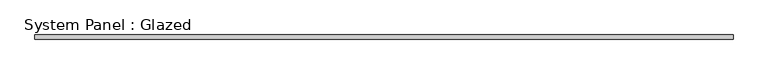
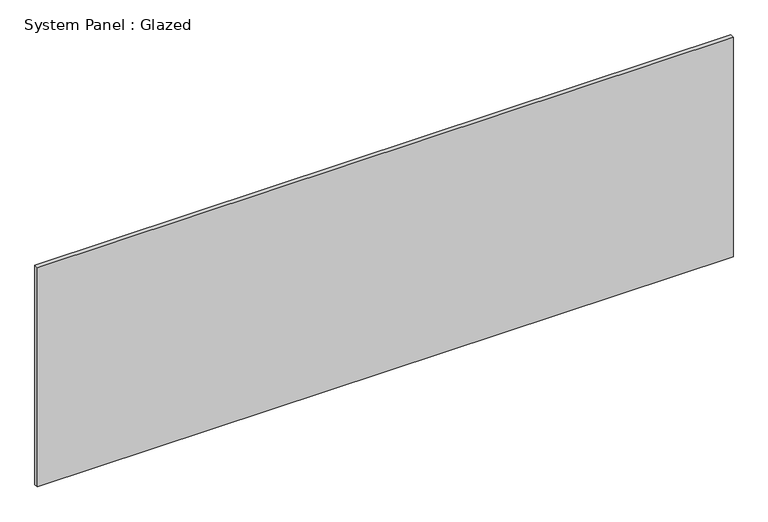
"""IFC4 building model written with IfcOpenShell, lengths in millimetres: plate geometry, System Panel : Glazed."""

from ifc_helpers import new_model, si_unit, origin, origin_with_axes, place, context, project, spatial, polyline, outline, extrude, source, transform, mapped, element, save


def system_panel_glazed_4ec28fe5(model_context):
    return source(origin(), model_context, "Body", "SweptSolid", [
        extrude(outline(polyline([(2146.3, 19.05), (-2146.3, 19.05), (-2146.3, 44.45), (2146.3, 44.45), (2146.3, 19.05)])), origin_with_axes(), (0.0, 0.0, 1.0), 1430.0433028),
    ])


if __name__ == "__main__":
    model = new_model("IFC4")
    model_context = context("Model", 3, world=origin())
    ifc_project = project(units=[si_unit("LENGTHUNIT", "METRE", prefix="MILLI")], contexts=[model_context])
    site = spatial("IfcSite", under=ifc_project)
    building = spatial("IfcBuilding", under=site)
    placement = place(None, origin())
    system_panel_glazed_shape = system_panel_glazed_4ec28fe5(model_context)
    element("IfcPlate", 1, ObjectType="System Panel : Glazed", at=placement, inside=building, context=model_context, shape_type="MappedRepresentation", body=[
        mapped(system_panel_glazed_shape, transform((0.0, 0.0, 0.0), x_axis=(1.0, 0.0, 0.0), y_axis=(0.0, 1.0, 0.0), z_axis=(0.0, 0.0, 1.0))),
    ])
    save(model, "model.ifc")

# Revit data of these elements
# Type "System Panel : Glazed"
#   Construction Type Id = "GSP4R"
#   Analytic Construction = "1/8 in Pilkington single glazing"
#   Visual Light Transmittance = 0.9
#   Solar Heat Gain Coefficient = 0.86
#   Heat Transfer Coefficient (U) = 1.18115 BTU/(h·ft²·°F)
#   Define Thermal Properties by = 1
# Element 1 (IfcPlate, "System Panel : Glazed")
#   Materials on its faces: "Glass"
# Materials
#   "Glass": class "Glass", colour RGB 0 128 192, transparency 0.75, Description = "Soda Lime Glass", Cost = 0
